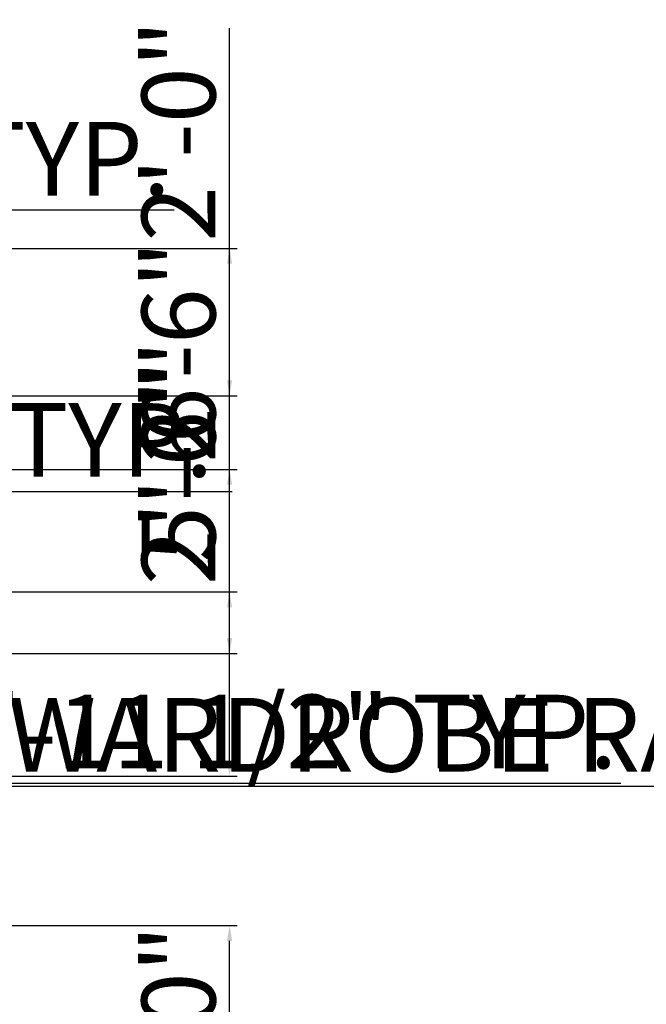
# Model space of a CAD drawing. Units: millimetres. Extents: x 542930 to 543750, y 628093 to 628738.
# Tile 12 of 14: x 543502 to 543604, y 628458 to 628618. Entities that reach past the tile are written whole.
import ezdxf

# ---------------------------------------------------------------- set-up
doc = ezdxf.new("R2010")
doc.units = ezdxf.units.MM
doc.layers.add('A-ANNO-DIMS', color=2, linetype='Continuous', lineweight=18)
doc.styles.get("Standard").update_dxf_attribs({"font": 'arial.ttf'})
doc.dimstyles.new('ISO-25', dxfattribs={"dimtxt": 12, "dimasz": 2.5, "dimexe": 1.25, "dimexo": 0.625, "dimtad": 1, "dimdec": 0, "dimlunit": 3, "dimtxsty": 'Standard', "dimcen": 2.5, "dimadec": 0, "dimazin": 0, "dimtfac": 1, "dimtdec": 0, "dimtmove": 0, "dimatfit": 3, "dimfxl": 1, "dimarcsym": 0})

# ---------------------------------------------------------------- blocks, each defined once
blk = doc.blocks.new('*D36')
at = {"layer": 'A-ANNO-DIMS', "color": 0, "lineweight": -2, "transparency": 16777216}
for p, q in [((543474.49, 628495.22), (543474.49, 628492.48)), ((543476.99, 628493.73), (543483.58, 628493.73)), ((543486.08, 628495.22), (543486.08, 628492.48)), ((543486.08, 628493.73), (543600.26, 628493.73))]:
    blk.add_line(p, q, dxfattribs=at)
at = {"layer": 'A-ANNO-DIMS', "color": 0, "transparency": 16777216}
for points in [[(543476.99, 628494.14), (543476.99, 628493.31), (543474.49, 628493.73)], [(543483.58, 628494.14), (543483.58, 628493.31), (543486.08, 628493.73)]]:
    blk.add_solid(points, dxfattribs=at)
at = {"layer": 'Defpoints', "color": 0, "transparency": 16777216}
for p in [(543474.49, 628495.85), (543486.08, 628495.85), (543486.08, 628493.73)]:
    blk.add_point(p, dxfattribs=at)
at = {"layer": 'A-ANNO-DIMS', "color": 0, "transparency": 16777216, "insert": (543544.42, 628500.56), "char_height": 12, "attachment_point": 5}
blk.add_mtext('0\'-11 1/2" TYP.', dxfattribs=at)
blk = doc.blocks.new('*D45')
at = {"layer": 'A-ANNO-DIMS', "color": 0, "lineweight": -2, "transparency": 16777216}
for p, q in [((543407.17, 628481.45), (543407.17, 628494.45)), ((543489.67, 628481.45), (543489.67, 628494.45)), ((543409.67, 628493.2), (543487.17, 628493.2)), ((543489.67, 628493.2), (543749.65, 628493.2))]:
    blk.add_line(p, q, dxfattribs=at)
at = {"layer": 'A-ANNO-DIMS', "color": 0, "transparency": 16777216}
for points in [[(543409.67, 628493.62), (543409.67, 628492.78), (543407.17, 628493.2)], [(543487.17, 628493.62), (543487.17, 628492.78), (543489.67, 628493.2)]]:
    blk.add_solid(points, dxfattribs=at)
at = {"layer": 'Defpoints', "color": 0, "transparency": 16777216}
for p in [(543489.67, 628493.2), (543407.17, 628480.83), (543489.67, 628480.83)]:
    blk.add_point(p, dxfattribs=at)
at = {"layer": 'A-ANNO-DIMS', "color": 0, "transparency": 16777216, "insert": (543620.91, 628500.03), "char_height": 12, "attachment_point": 5}
blk.add_mtext('WARDROBE RAIL 6\'-10 1/2" TYP.', dxfattribs=at)
blk = doc.blocks.new('*D54')
at = {"layer": 'A-ANNO-DIMS', "color": 0, "lineweight": -2, "transparency": 16777216}
for p, q in [((543414.67, 628581.45), (543414.67, 628588.38)), ((543450.67, 628581.45), (543450.67, 628588.38)), ((543417.17, 628587.13), (543448.17, 628587.13)), ((543450.67, 628587.13), (543527.55, 628587.13))]:
    blk.add_line(p, q, dxfattribs=at)
at = {"layer": 'A-ANNO-DIMS', "color": 0, "transparency": 16777216}
for points in [[(543417.17, 628587.54), (543417.17, 628586.71), (543414.67, 628587.13)], [(543448.17, 628587.54), (543448.17, 628586.71), (543450.67, 628587.13)]]:
    blk.add_solid(points, dxfattribs=at)
at = {"layer": 'Defpoints', "color": 0, "transparency": 16777216}
for p in [(543450.67, 628587.13), (543414.67, 628580.83), (543450.67, 628580.83)]:
    blk.add_point(p, dxfattribs=at)
at = {"layer": 'A-ANNO-DIMS', "color": 0, "transparency": 16777216, "insert": (543490.36, 628593.88), "char_height": 12, "attachment_point": 5}
blk.add_mtext('3\'-0" TYP.', dxfattribs=at)
blk = doc.blocks.new('*D57')
at = {"layer": 'A-ANNO-DIMS', "color": 0, "lineweight": -2, "transparency": 16777216}
for p, q in [((543374.67, 628544.2), (543374.67, 628539.98)), ((543398.67, 628544.2), (543398.67, 628539.98)), ((543377.17, 628541.23), (543396.17, 628541.23)), ((543398.67, 628541.23), (543536.99, 628541.23))]:
    blk.add_line(p, q, dxfattribs=at)
at = {"layer": 'A-ANNO-DIMS', "color": 0, "transparency": 16777216}
for points in [[(543377.17, 628541.64), (543377.17, 628540.81), (543374.67, 628541.23)], [(543396.17, 628541.64), (543396.17, 628540.81), (543398.67, 628541.23)]]:
    blk.add_solid(points, dxfattribs=at)
at = {"layer": 'Defpoints', "color": 0, "transparency": 16777216}
for p in [(543374.67, 628544.83), (543398.67, 628544.83), (543398.67, 628541.23)]:
    blk.add_point(p, dxfattribs=at)
at = {"layer": 'A-ANNO-DIMS', "color": 0, "transparency": 16777216, "insert": (543469.08, 628548.06), "char_height": 12, "attachment_point": 5}
blk.add_mtext('STOOL 2\'-0" TYP.', dxfattribs=at)
blk = doc.blocks.new('*D70')
at = {"layer": 'A-ANNO-DIMS', "color": 0, "lineweight": -2, "transparency": 16777216}
for p, q in [((543325.79, 628580.83), (543537.81, 628580.83)), ((543536.56, 628517.33), (543536.56, 628578.33)), ((543325.79, 628514.83), (543537.81, 628514.83))]:
    blk.add_line(p, q, dxfattribs=at)
at = {"layer": 'A-ANNO-DIMS', "color": 0, "transparency": 16777216}
for points in [[(543536.15, 628578.33), (543536.98, 628578.33), (543536.56, 628580.83)], [(543536.15, 628517.33), (543536.98, 628517.33), (543536.56, 628514.83)]]:
    blk.add_solid(points, dxfattribs=at)
at = {"layer": 'Defpoints', "color": 0, "transparency": 16777216}
for p in [(543325.17, 628580.83), (543536.56, 628580.83), (543325.17, 628514.83)]:
    blk.add_point(p, dxfattribs=at)
at = {"layer": 'A-ANNO-DIMS', "color": 0, "transparency": 16777216, "insert": (543529.81, 628547.83), "char_height": 12, "attachment_point": 5, "rotation": 90}
blk.add_mtext('5\'-6"', dxfattribs=at)
blk = doc.blocks.new('*D72')
at = {"layer": 'A-ANNO-DIMS', "color": 0, "lineweight": -2, "transparency": 16777216}
for p, q in [((543536.56, 628544.83), (543536.56, 628580.68)), ((543282.29, 628544.83), (543537.81, 628544.83)), ((543536.56, 628517.33), (543536.56, 628542.33)), ((543282.29, 628514.83), (543537.81, 628514.83))]:
    blk.add_line(p, q, dxfattribs=at)
at = {"layer": 'A-ANNO-DIMS', "color": 0, "transparency": 16777216}
for points in [[(543536.15, 628542.33), (543536.98, 628542.33), (543536.56, 628544.83)], [(543536.15, 628517.33), (543536.98, 628517.33), (543536.56, 628514.83)]]:
    blk.add_solid(points, dxfattribs=at)
at = {"layer": 'Defpoints', "color": 0, "transparency": 16777216}
for p in [(543281.67, 628544.83), (543536.56, 628544.83), (543281.67, 628514.83)]:
    blk.add_point(p, dxfattribs=at)
at = {"layer": 'A-ANNO-DIMS', "color": 0, "transparency": 16777216, "insert": (543529.81, 628564), "char_height": 12, "attachment_point": 5, "rotation": 90}
blk.add_mtext('2\'-6"', dxfattribs=at)
blk = doc.blocks.new('*D77')
at = {"layer": 'A-ANNO-DIMS', "color": 0, "lineweight": -2, "transparency": 16777216}
for p, q in [((543536.56, 628524.86), (543536.56, 628560.72)), ((543415.29, 628524.86), (543537.81, 628524.86)), ((543536.56, 628497.36), (543536.56, 628522.36)), ((543415.29, 628494.86), (543537.81, 628494.86))]:
    blk.add_line(p, q, dxfattribs=at)
at = {"layer": 'A-ANNO-DIMS', "color": 0, "transparency": 16777216}
for points in [[(543536.15, 628522.36), (543536.98, 628522.36), (543536.56, 628524.86)], [(543536.15, 628497.36), (543536.98, 628497.36), (543536.56, 628494.86)]]:
    blk.add_solid(points, dxfattribs=at)
at = {"layer": 'Defpoints', "color": 0, "transparency": 16777216}
for p in [(543414.67, 628524.86), (543536.56, 628524.86), (543414.67, 628494.86)]:
    blk.add_point(p, dxfattribs=at)
at = {"layer": 'A-ANNO-DIMS', "color": 0, "transparency": 16777216, "insert": (543529.81, 628544.04), "char_height": 12, "attachment_point": 5, "rotation": 90}
blk.add_mtext('2\'-6"', dxfattribs=at)
blk = doc.blocks.new('*D80')
at = {"layer": 'A-ANNO-DIMS', "color": 0, "lineweight": -2, "transparency": 16777216}
for p, q in [((543228.79, 628470.52), (543537.81, 628470.52)), ((543536.56, 628437.09), (543536.56, 628468.02)), ((543228.79, 628434.59), (543537.81, 628434.59))]:
    blk.add_line(p, q, dxfattribs=at)
at = {"layer": 'A-ANNO-DIMS', "color": 0, "transparency": 16777216}
for points in [[(543536.15, 628468.02), (543536.98, 628468.02), (543536.56, 628470.52)], [(543536.15, 628437.09), (543536.98, 628437.09), (543536.56, 628434.59)]]:
    blk.add_solid(points, dxfattribs=at)
at = {"layer": 'Defpoints', "color": 0, "transparency": 16777216}
for p in [(543228.16, 628470.52), (543536.56, 628470.52), (543228.16, 628434.59)]:
    blk.add_point(p, dxfattribs=at)
at = {"layer": 'A-ANNO-DIMS', "color": 0, "transparency": 16777216, "insert": (543529.81, 628452.55), "char_height": 12, "attachment_point": 5, "rotation": 90}
blk.add_mtext('3\'-0"', dxfattribs=at)
blk = doc.blocks.new('*D83')
at = {"layer": 'A-ANNO-DIMS', "color": 0, "lineweight": -2, "transparency": 16777216}
for p, q in [((543536.56, 628580.83), (543536.56, 628616.68)), ((543410.79, 628580.83), (543537.81, 628580.83)), ((543536.56, 628559.33), (543536.56, 628578.33)), ((543410.79, 628556.83), (543537.81, 628556.83))]:
    blk.add_line(p, q, dxfattribs=at)
at = {"layer": 'A-ANNO-DIMS', "color": 0, "transparency": 16777216}
for points in [[(543536.15, 628578.33), (543536.98, 628578.33), (543536.56, 628580.83)], [(543536.15, 628559.33), (543536.98, 628559.33), (543536.56, 628556.83)]]:
    blk.add_solid(points, dxfattribs=at)
at = {"layer": 'Defpoints', "color": 0, "transparency": 16777216}
for p in [(543410.17, 628580.83), (543536.56, 628580.83), (543410.17, 628556.83)]:
    blk.add_point(p, dxfattribs=at)
at = {"layer": 'A-ANNO-DIMS', "color": 0, "transparency": 16777216, "insert": (543529.81, 628600), "char_height": 12, "attachment_point": 5, "rotation": 90}
blk.add_mtext('2\'-0"', dxfattribs=at)

msp = doc.modelspace()

# ---------------------------------------------------------------- dimensions: what is measured, and where the dimension line sits
at = {"layer": 'A-ANNO-DIMS'}
for base, p1, p2, picture, middle in [((543536.56, 628580.83), (543410.17, 628556.83), (543410.17, 628580.83), '*D83', (543529.81, 628600)), ((543536.56, 628544.83), (543281.67, 628514.83), (543281.67, 628544.83), '*D72', (543529.81, 628564)), ((543536.56, 628580.83), (543325.17, 628514.83), (543325.17, 628580.83), '*D70', (543529.81, 628547.83)), ((543536.56, 628524.86), (543414.67, 628494.86), (543414.67, 628524.86), '*D77', (543529.81, 628544.04)), ((543536.56, 628470.52), (543228.16, 628434.59), (543228.16, 628470.52), '*D80', (543529.81, 628452.55))]:
    dim = msp.add_linear_dim(base=base, p1=p1, p2=p2, angle=90, dimstyle='ISO-25', override={"dimdec": 1, "dimlfac": 1, "dimrnd": 0, "dimzin": 1, "dimdsep": 46, "dimlunit": 4, "dimfrac": 2}, dxfattribs=at)
    dim.commit()
    dim.dimension.update_dxf_attribs({"geometry": picture, "text_midpoint": middle})
for base, p1, p2, text, picture, middle in [((543450.67, 628587.13), (543414.67, 628580.83), (543450.67, 628580.83), '<> TYP.', '*D54', (543490.36, 628593.88)), ((543398.67, 628541.23), (543374.67, 628544.83), (543398.67, 628544.83), 'STOOL <> TYP.', '*D57', (543469.08, 628548.06)), ((543489.67, 628493.2), (543407.17, 628480.83), (543489.67, 628480.83), 'WARDROBE RAIL <> TYP.', '*D45', (543620.91, 628500.03)), ((543486.08, 628493.73), (543474.49, 628495.85), (543486.08, 628495.85), '<> TYP.', '*D36', (543544.42, 628500.56))]:
    dim = msp.add_linear_dim(base=base, p1=p1, p2=p2, text=text, dimstyle='ISO-25', override={"dimdec": 1, "dimlfac": 1, "dimrnd": 0, "dimzin": 1, "dimdsep": 46, "dimlunit": 4, "dimfrac": 2}, dxfattribs=at)
    dim.commit()
    dim.dimension.update_dxf_attribs({"geometry": picture, "text_midpoint": middle})

doc.saveas('drawing.dxf')
